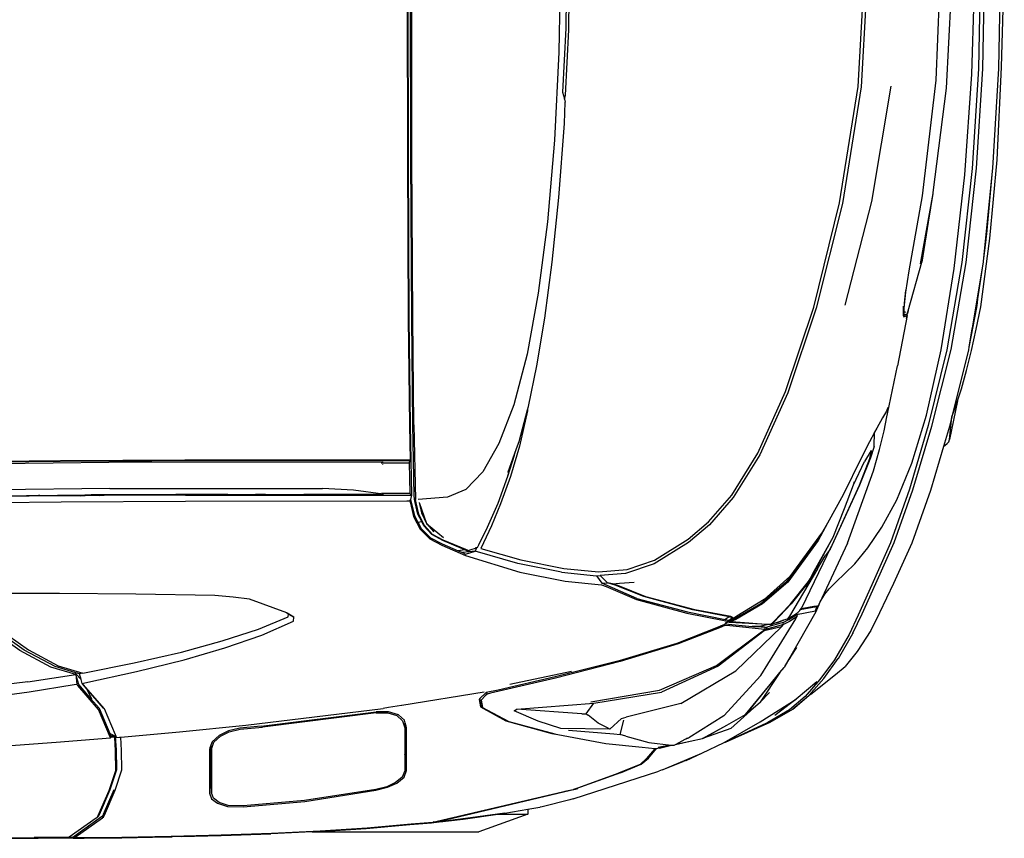
# Model space of a CAD drawing. Units: inches. Extents: x 22042254 to 25404563, y 17568978 to 17626777.
# Tile 7 of 45: x 22042256.1597 to 22042256.7839, y 17568977.6632 to 17568978.1821. Entities that reach past the tile are written whole.
import ezdxf

# ---------------------------------------------------------------- set-up
doc = ezdxf.new("R2010")
doc.units = ezdxf.units.IN
doc.header["$MEASUREMENT"] = 0
doc.layers.add('A-SITE-VEHI', color=8, linetype='Continuous', lineweight=18)
doc.layers.add('Edges', color=250, linetype='Continuous')

# ---------------------------------------------------------------- blocks, each defined once
blk = doc.blocks.new('Nissan Qashqai pl')
at = {"layer": 'Edges'}
for p, q in [((10.6151, 12.8159), (10.6644, 12.8162)), ((10.6176, 12.8164), (10.6651, 12.8167)), ((10.6644, 12.8162), (10.7078, 12.8159)), ((10.6651, 12.8167), (10.666, 12.8167)), ((10.666, 12.8167), (10.677, 12.8167)), ((10.6729, 12.8157), (10.7082, 12.8156)), ((10.6809, 12.8167), (10.677, 12.8167)), ((10.7128, 12.8166), (10.6809, 12.8167)), ((10.7078, 12.8159), (10.7083, 12.8156)), ((10.7082, 12.8156), (10.7078, 12.8159)), ((10.7085, 12.8153), (10.7082, 12.8156)), ((10.7082, 12.8156), (10.7083, 12.8156)), ((10.7083, 12.8156), (10.7087, 12.8153)), ((10.7083, 12.8156), (10.7125, 12.8156)), ((10.7087, 12.8153), (10.7363, 12.7959)), ((10.7139, 12.8164), (10.7125, 12.8156)), ((10.7137, 12.8148), (10.7125, 12.8156)), ((10.7128, 12.8166), (10.7625, 12.8161)), ((10.7128, 12.8166), (10.724, 12.8166)), ((10.7139, 12.8164), (10.7148, 12.8157)), ((10.7628, 12.8158), (10.7139, 12.8164)), ((10.7148, 12.8157), (10.7429, 12.7956)), ((10.7685, 12.8161), (10.724, 12.8166)), ((10.7625, 12.8161), (10.7628, 12.8161)), ((10.7628, 12.8161), (10.8099, 12.8152)), ((10.8131, 12.8149), (10.7628, 12.8158)), ((10.7688, 12.8161), (10.7685, 12.8161)), ((10.8099, 12.8152), (10.7688, 12.8161)), ((10.8099, 12.8152), (10.8131, 12.8152)), ((10.8134, 12.8152), (10.8131, 12.8152)), ((10.8134, 12.8152), (10.8142, 12.8152)), ((10.8142, 12.8152), (10.8142, 12.8152)), ((10.8237, 12.8149), (10.8142, 12.8152)), ((10.7137, 12.8148), (10.7138, 12.8147)), ((10.7418, 12.7947), (10.7138, 12.8147)), ((10.8644, 12.8135), (10.8131, 12.8149)), ((10.8237, 12.8149), (10.864, 12.8138)), ((10.8596, 12.8138), (10.8589, 12.8138)), ((10.8642, 12.8136), (10.8596, 12.8138)), ((10.864, 12.8138), (10.8642, 12.8138)), ((10.8642, 12.8138), (10.9152, 12.812)), ((10.9158, 12.8118), (10.8644, 12.8135)), ((10.9577, 12.8101), (10.9152, 12.812)), ((10.9657, 12.8095), (10.9158, 12.8118)), ((10.9577, 12.8101), (10.9649, 12.8097)), ((10.9577, 12.8101), (11.1283, 12.8101)), ((10.9649, 12.8097), (11.0127, 12.8067)), ((11.0138, 12.8064), (10.9657, 12.8095)), ((11.0127, 12.8067), (11.0576, 12.8026)), ((11.059, 12.8023), (11.0138, 12.8064)), ((11.1783, 12.7921), (11.1283, 12.8101)), ((10.7363, 12.7959), (10.7376, 12.795)), ((10.7387, 12.794), (10.7376, 12.795)), ((10.7376, 12.795), (10.7378, 12.7946)), ((10.7432, 12.7954), (10.7426, 12.7954)), ((10.7429, 12.7956), (10.7432, 12.7954)), ((10.7441, 12.7954), (10.7432, 12.7954)), ((10.7432, 12.7954), (10.744, 12.7948)), ((11.0576, 12.8026), (11.0798, 12.8008)), ((11.0768, 12.8008), (11.059, 12.8023)), ((11.0811, 12.8004), (11.0768, 12.8008)), ((11.0798, 12.8008), (11.0872, 12.7999)), ((11.0827, 12.8001), (11.0811, 12.8004)), ((11.0827, 12.8001), (11.0813, 12.7998)), ((11.0836, 12.8002), (11.0827, 12.8001)), ((11.0856, 12.7994), (11.0827, 12.8001)), ((11.0872, 12.7999), (11.0836, 12.8002)), ((11.0836, 12.8002), (11.0882, 12.7992)), ((11.2196, 12.7681), (11.0856, 12.7994)), ((11.0883, 12.7998), (11.0872, 12.7999)), ((11.0882, 12.7992), (11.2222, 12.7676)), ((11.0883, 12.7998), (11.1123, 12.797)), ((11.1147, 12.7965), (11.0883, 12.7998)), ((11.1123, 12.797), (11.1475, 12.7921)), ((11.1547, 12.791), (11.1147, 12.7965)), ((10.7378, 12.7946), (10.7379, 12.7945)), ((10.7378, 12.7946), (10.7385, 12.7932)), ((10.7385, 12.7932), (10.7497, 12.7679)), ((10.7387, 12.794), (10.7396, 12.7922)), ((10.7396, 12.7922), (10.7507, 12.7669)), ((10.743, 12.7939), (10.7418, 12.7947)), ((10.7434, 12.793), (10.743, 12.7939)), ((10.7437, 12.7921), (10.7434, 12.793)), ((10.7438, 12.7921), (10.7437, 12.7921)), ((10.7438, 12.7921), (10.7549, 12.7666)), ((10.744, 12.7948), (10.7448, 12.793)), ((10.7448, 12.793), (10.7559, 12.7674)), ((11.1475, 12.7921), (11.1525, 12.7914)), ((11.1475, 12.7921), (11.1783, 12.7921)), ((11.1525, 12.7914), (11.1547, 12.791)), ((11.1547, 12.791), (11.1783, 12.787)), ((11.1783, 12.787), (11.1783, 12.7921)), ((11.1783, 12.787), (11.1906, 12.7849)), ((11.1906, 12.7849), (11.1909, 12.7849)), ((11.193, 12.7845), (11.1909, 12.7849)), ((10.8523, 12.7704), (10.8546, 12.7762)), ((10.8565, 12.7757), (10.8543, 12.7702)), ((10.8546, 12.7762), (10.8607, 12.7808)), ((10.8622, 12.7801), (10.8565, 12.7757)), ((10.8607, 12.7808), (10.8708, 12.7841)), ((10.8716, 12.7832), (10.8622, 12.7801)), ((10.8708, 12.7841), (10.8869, 12.7844)), ((10.887, 12.7835), (10.8716, 12.7832)), ((10.8869, 12.7844), (10.9499, 12.7789)), ((10.9498, 12.7781), (10.887, 12.7835)), ((11.0226, 12.7668), (10.9498, 12.7781)), ((10.9499, 12.7789), (11.0229, 12.7676)), ((11.2215, 12.7775), (11.193, 12.7845)), ((11.2247, 12.7764), (11.2215, 12.7775)), ((11.2247, 12.7764), (11.3124, 12.7479)), ((10.7497, 12.7679), (10.7565, 12.7473)), ((10.7507, 12.7669), (10.7575, 12.7462)), ((10.7559, 12.7674), (10.7626, 12.7467)), ((10.8523, 12.7255), (10.8523, 12.7704)), ((10.8543, 12.7702), (10.8538, 12.753)), ((10.8543, 12.7255), (10.8543, 12.7702)), ((11.0339, 12.7639), (11.0226, 12.7668)), ((11.0229, 12.7676), (11.0348, 12.7645)), ((11.2247, 12.767), (11.2163, 12.7689)), ((11.22, 12.768), (11.2196, 12.7681)), ((11.2247, 12.767), (11.22, 12.768)), ((11.2222, 12.7676), (11.2271, 12.7664)), ((11.2253, 12.7668), (11.2247, 12.767)), ((11.2304, 12.7649), (11.2253, 12.7668)), ((11.2253, 12.7668), (11.2271, 12.7664)), ((11.2271, 12.7664), (11.2296, 12.7658)), ((11.2271, 12.7664), (11.2277, 12.7662)), ((11.2277, 12.7662), (11.2296, 12.7658)), ((11.2732, 12.7496), (11.2277, 12.7662)), ((11.2704, 12.7504), (11.2304, 12.7649)), ((11.0429, 12.7597), (11.0339, 12.7639)), ((11.0348, 12.7645), (11.0444, 12.7601)), ((11.0497, 12.7542), (11.0429, 12.7597)), ((11.0444, 12.7601), (11.0516, 12.7542)), ((10.7565, 12.7473), (10.7563, 12.7273)), ((10.7575, 12.7462), (10.7572, 12.7263)), ((10.7626, 12.7467), (10.7623, 12.7269)), ((10.8528, 12.7503), (10.8535, 12.7521)), ((10.8528, 12.742), (10.8528, 12.7503)), ((10.8535, 12.7521), (10.8538, 12.753)), ((10.8538, 12.7521), (10.8535, 12.7521)), ((10.8538, 12.753), (10.8538, 12.7521)), ((10.8538, 12.7521), (10.8538, 12.7502)), ((10.8538, 12.7502), (10.8538, 12.742)), ((11.0523, 12.7475), (11.0497, 12.7542)), ((11.0516, 12.7542), (11.0543, 12.7473)), ((11.0528, 12.73), (11.0523, 12.7475)), ((11.0523, 12.7312), (11.0523, 12.7475)), ((11.0543, 12.7473), (11.0543, 12.7035)), ((11.2702, 12.7507), (11.2704, 12.7504)), ((11.2704, 12.7506), (11.2707, 12.7503)), ((11.2707, 12.7503), (11.2704, 12.7504)), ((11.2719, 12.7498), (11.2707, 12.7503)), ((11.2934, 12.741), (11.2719, 12.7498)), ((11.2732, 12.7496), (11.2946, 12.7409)), ((11.3161, 12.7467), (11.3124, 12.7479)), ((11.3161, 12.7467), (11.3376, 12.7381)), ((11.3192, 12.7454), (11.3566, 12.7294)), ((10.8528, 12.742), (10.8538, 12.742)), ((10.8528, 12.7419), (10.8528, 12.742)), ((10.8538, 12.7419), (10.8528, 12.7419)), ((10.8528, 12.7242), (10.8528, 12.7419)), ((10.8538, 12.742), (10.8538, 12.7419)), ((10.8538, 12.7214), (10.8538, 12.7419)), ((11.3, 12.735), (11.2934, 12.741)), ((11.2946, 12.7409), (11.3018, 12.7346)), ((11.3081, 12.7253), (11.3, 12.735)), ((11.3018, 12.7346), (11.3103, 12.7249)), ((11.3405, 12.7369), (11.3376, 12.7381)), ((11.3405, 12.7369), (11.3566, 12.7294)), ((10.7563, 12.7273), (10.7553, 12.7134)), ((10.7572, 12.7263), (10.7563, 12.7126)), ((10.7623, 12.7269), (10.7615, 12.7131)), ((10.8528, 12.7242), (10.8523, 12.7255)), ((10.8543, 12.7255), (10.8569, 12.7184)), ((11.0523, 12.7312), (11.0528, 12.73)), ((11.0523, 12.7287), (11.0523, 12.7312)), ((11.0528, 12.7274), (11.0523, 12.7287)), ((11.0523, 12.7037), (11.0523, 12.7287)), ((11.0528, 12.7274), (11.0528, 12.73)), ((11.0528, 12.73), (11.0538, 12.7273)), ((11.0528, 12.7274), (11.0528, 12.6985)), ((11.0538, 12.7273), (11.0538, 12.7018)), ((11.2956, 12.7234), (11.3085, 12.7247)), ((11.3086, 12.7247), (11.3081, 12.7253)), ((11.3081, 12.7253), (11.3087, 12.7247)), ((11.3085, 12.7247), (11.3086, 12.7247)), ((11.3086, 12.7247), (11.3087, 12.7247)), ((11.3087, 12.7247), (11.3103, 12.7249)), ((11.3103, 12.7249), (11.3103, 12.7249)), ((11.3103, 12.7249), (11.3106, 12.7249)), ((11.3106, 12.7249), (11.314, 12.7238)), ((11.3566, 12.7294), (11.3796, 12.7187)), ((10.6318, 12.7228), (10.6955, 12.7184)), ((10.6955, 12.7184), (10.7509, 12.714)), ((10.8538, 12.7214), (10.8528, 12.7242)), ((10.855, 12.7181), (10.8538, 12.7214)), ((10.8622, 12.7114), (10.855, 12.7181)), ((10.8569, 12.7184), (10.8637, 12.712)), ((11.2091, 12.7103), (11.2583, 12.7196)), ((11.2583, 12.7196), (11.2956, 12.7234)), ((11.2787, 12.7123), (11.3022, 12.7186)), ((11.3022, 12.7186), (11.3252, 12.7213)), ((11.317, 12.7227), (11.3119, 12.7236)), ((11.3132, 12.7243), (11.3256, 12.7215)), ((11.314, 12.7238), (11.317, 12.7227)), ((11.314, 12.7238), (11.3242, 12.7216)), ((11.3242, 12.7216), (11.317, 12.7227)), ((11.3198, 12.7211), (11.3252, 12.7213)), ((11.3242, 12.7216), (11.3256, 12.7215)), ((11.3252, 12.7213), (11.3283, 12.7214)), ((11.3256, 12.7215), (11.3283, 12.7214)), ((11.3283, 12.7214), (11.3297, 12.7206)), ((11.3297, 12.7206), (11.3446, 12.7173)), ((11.3297, 12.7206), (11.3302, 12.7203)), ((11.3302, 12.7203), (11.3446, 12.7173)), ((11.3302, 12.7203), (11.3394, 12.7152)), ((11.3394, 12.7152), (11.3434, 12.7138)), ((11.3394, 12.7152), (11.342, 12.7137)), ((11.3446, 12.7173), (11.3571, 12.7146)), ((11.3583, 12.7142), (11.3571, 12.7146)), ((11.3571, 12.7146), (11.3821, 12.7008)), ((11.3796, 12.7187), (11.4164, 12.6974)), ((11.3796, 12.7187), (11.3807, 12.7182)), ((11.3807, 12.7182), (11.4267, 12.6979)), ((11.4228, 12.6989), (11.3807, 12.7182)), ((10.7501, 12.7114), (10.7387, 12.6849)), ((10.7507, 12.7098), (10.7397, 12.684)), ((10.7563, 12.7109), (10.7449, 12.6843)), ((10.7507, 12.7132), (10.7501, 12.7114)), ((10.7506, 12.7111), (10.7507, 12.7132)), ((10.7507, 12.7132), (10.7509, 12.714)), ((10.751, 12.7132), (10.7507, 12.7132)), ((10.7511, 12.7107), (10.7507, 12.7098)), ((10.7524, 12.7106), (10.7507, 12.7098)), ((10.7522, 12.7131), (10.7509, 12.714)), ((10.7516, 12.7131), (10.7509, 12.714)), ((10.7519, 12.7128), (10.7511, 12.7107)), ((10.7522, 12.7131), (10.7516, 12.7131)), ((10.7519, 12.7128), (10.7516, 12.7131)), ((10.7526, 12.7124), (10.7519, 12.7128)), ((10.7553, 12.7134), (10.7522, 12.7131)), ((10.7524, 12.7106), (10.7526, 12.7124)), ((10.7556, 12.7122), (10.7524, 12.7106)), ((10.7526, 12.7124), (10.7526, 12.7127)), ((10.7532, 12.712), (10.7526, 12.7124)), ((10.7556, 12.7122), (10.7532, 12.712)), ((10.7561, 12.7125), (10.7556, 12.7122)), ((10.7561, 12.7125), (10.7563, 12.7126)), ((10.7563, 12.7125), (10.7561, 12.7125)), ((10.7563, 12.7123), (10.7561, 12.7123)), ((10.7563, 12.7126), (10.7573, 12.7135)), ((10.7563, 12.7126), (10.7563, 12.7125)), ((10.7569, 12.7125), (10.7563, 12.7109)), ((10.7569, 12.7125), (10.7563, 12.7125)), ((10.7563, 12.7125), (10.7563, 12.7123)), ((10.7573, 12.7135), (10.7569, 12.7125)), ((10.7573, 12.7135), (10.7604, 12.7132)), ((10.7604, 12.7132), (10.7615, 12.7131)), ((10.7615, 12.7131), (10.8218, 12.7077)), ((10.8218, 12.7077), (10.8896, 12.7008)), ((10.8718, 12.7068), (10.8622, 12.7114)), ((10.8637, 12.712), (10.8727, 12.7077)), ((10.8836, 12.7041), (10.8718, 12.7068)), ((10.8727, 12.7077), (10.8839, 12.7051)), ((10.8839, 12.7051), (10.9067, 12.7029)), ((11.156, 12.6966), (11.203, 12.7093)), ((11.1589, 12.6971), (11.2062, 12.7098)), ((11.2121, 12.7043), (11.189, 12.6968)), ((11.203, 12.7093), (11.2091, 12.7103)), ((11.2062, 12.7098), (11.2091, 12.7103)), ((11.2622, 12.7051), (11.2121, 12.7043)), ((11.2199, 12.706), (11.2666, 12.7097)), ((11.2622, 12.7051), (11.2601, 12.7037)), ((11.2743, 12.6942), (11.2622, 12.7051)), ((11.2666, 12.7097), (11.2729, 12.7104)), ((11.2787, 12.7123), (11.2729, 12.7104)), ((11.2729, 12.7104), (11.2766, 12.6957)), ((11.379, 12.6915), (11.3434, 12.7138)), ((11.3583, 12.7142), (11.3821, 12.7008)), ((11.3864, 12.7044), (11.3583, 12.7142)), ((11.4163, 12.6775), (11.3864, 12.7044)), ((10.9054, 12.702), (10.8836, 12.7041)), ((10.8896, 12.7008), (11.0304, 12.6838)), ((10.9054, 12.702), (11.0232, 12.6871)), ((11.0231, 12.6882), (10.9067, 12.7029)), ((11.0443, 12.6911), (11.0501, 12.6964)), ((11.052, 12.6958), (11.0458, 12.6903)), ((11.0501, 12.6964), (11.0523, 12.7037)), ((11.0528, 12.6985), (11.052, 12.6958)), ((11.0538, 12.7018), (11.0528, 12.6985)), ((11.0543, 12.7035), (11.0538, 12.7018)), ((11.1298, 12.6823), (11.156, 12.6966)), ((11.1365, 12.6851), (11.1589, 12.6971)), ((11.189, 12.6968), (11.1644, 12.6862)), ((11.2505, 12.6987), (11.2401, 12.6908)), ((11.2601, 12.7037), (11.2505, 12.6987)), ((11.2743, 12.6942), (11.2791, 12.6927)), ((11.3821, 12.7008), (11.4014, 12.69)), ((11.4164, 12.6974), (11.4531, 12.6744)), ((11.4243, 12.6982), (11.4228, 12.6989)), ((11.4464, 12.6853), (11.4243, 12.6982)), ((11.4267, 12.6979), (11.4498, 12.6844)), ((10.7387, 12.6849), (10.7177, 12.6604)), ((10.7449, 12.6843), (10.7232, 12.6594)), ((11.0231, 12.6882), (11.035, 12.6883)), ((11.0358, 12.6872), (11.0232, 12.6871)), ((11.035, 12.6883), (11.0443, 12.6911)), ((11.0458, 12.6903), (11.0358, 12.6872)), ((11.1319, 12.6827), (11.1365, 12.6851)), ((11.1644, 12.6862), (11.1672, 12.6844)), ((11.2337, 12.6892), (11.1672, 12.6844)), ((11.1672, 12.6844), (11.2459, 12.6785)), ((11.2337, 12.6892), (11.2382, 12.6892)), ((11.2382, 12.6892), (11.2401, 12.6908)), ((11.2382, 12.6892), (11.2459, 12.6785)), ((11.335, 12.6786), (11.2791, 12.6927)), ((11.379, 12.6915), (11.417, 12.6499)), ((11.4014, 12.69), (11.4022, 12.6894)), ((11.4014, 12.69), (11.4265, 12.6594)), ((11.4022, 12.6894), (11.4163, 12.6775)), ((11.4022, 12.6894), (11.4265, 12.6594)), ((11.4531, 12.6744), (11.4314, 12.6911)), ((11.4624, 12.6717), (11.4464, 12.6853)), ((11.4498, 12.6844), (11.4662, 12.6706)), ((11.4681, 12.6691), (11.4498, 12.6844)), ((10.6678, 12.6672), (10.6152, 12.674)), ((10.7334, 12.6766), (10.7186, 12.6593)), ((10.7438, 12.6836), (10.7265, 12.6635)), ((10.7265, 12.6635), (10.7316, 12.6741)), ((10.7397, 12.684), (10.7334, 12.6766)), ((11.0357, 12.6829), (11.0304, 12.6838)), ((11.0491, 12.6807), (11.0357, 12.6829)), ((11.0449, 12.6812), (11.0448, 12.6812)), ((11.0492, 12.6807), (11.0491, 12.6807)), ((11.1336, 12.667), (11.0492, 12.6807)), ((11.1285, 12.6745), (11.1298, 12.6823)), ((11.1293, 12.6736), (11.1285, 12.6745)), ((11.1306, 12.6812), (11.1293, 12.6736)), ((11.1306, 12.6752), (11.1319, 12.6827)), ((11.1319, 12.6827), (11.1306, 12.6812)), ((11.1347, 12.671), (11.1306, 12.6752)), ((11.2428, 12.6769), (11.3132, 12.6652)), ((11.2459, 12.6785), (11.3153, 12.6672)), ((11.335, 12.6786), (11.3915, 12.6453)), ((11.4366, 12.6471), (11.4163, 12.6775)), ((11.4163, 12.6775), (11.4259, 12.6674)), ((11.4742, 12.6567), (11.4531, 12.6744)), ((10.7137, 12.6595), (10.6678, 12.6672)), ((11.1353, 12.6677), (11.1293, 12.6736)), ((11.1366, 12.6691), (11.1347, 12.671)), ((11.1358, 12.6676), (11.1353, 12.6677)), ((11.1358, 12.6676), (11.1366, 12.6691)), ((11.148, 12.665), (11.1358, 12.6676)), ((11.1401, 12.6682), (11.1366, 12.6691)), ((11.2066, 12.6527), (11.1401, 12.6682)), ((11.2063, 12.6515), (11.148, 12.665)), ((11.3132, 12.6652), (11.3715, 12.6398)), ((11.3733, 12.6404), (11.3153, 12.6672)), ((11.4774, 12.6543), (11.4624, 12.6717)), ((11.4662, 12.6706), (11.4815, 12.6531)), ((11.4681, 12.6691), (11.4936, 12.6491)), ((10.6664, 12.6566), (10.6144, 12.6629)), ((10.6664, 12.6566), (10.7155, 12.649)), ((10.7165, 12.6591), (10.7137, 12.6595)), ((10.7186, 12.6593), (10.7155, 12.649)), ((10.7155, 12.649), (10.7165, 12.6591)), ((10.7209, 12.654), (10.7155, 12.6485)), ((10.7177, 12.6604), (10.7165, 12.6591)), ((10.7209, 12.654), (10.7192, 12.6484)), ((10.7221, 12.6581), (10.7209, 12.654)), ((10.7232, 12.6594), (10.7221, 12.6581)), ((10.7221, 12.6581), (10.7224, 12.6587)), ((10.7221, 12.6581), (10.7247, 12.6575)), ((10.7265, 12.6635), (10.7224, 12.6587)), ((10.7247, 12.6575), (10.7776, 12.646)), ((11.2232, 12.6458), (11.1598, 12.6594)), ((11.4265, 12.6594), (11.4366, 12.6471)), ((11.4924, 12.6339), (11.4774, 12.6543)), ((10.7155, 12.649), (10.69, 12.6414)), ((10.7155, 12.6473), (10.6943, 12.641)), ((10.6976, 12.6401), (10.7228, 12.6477)), ((10.7155, 12.649), (10.7155, 12.6485)), ((10.7155, 12.6485), (10.7155, 12.6473)), ((10.7192, 12.6484), (10.7155, 12.6473)), ((10.7228, 12.6477), (10.7192, 12.6484)), ((10.7228, 12.6477), (10.7754, 12.637)), ((10.7776, 12.646), (10.8264, 12.6341)), ((11.272, 12.6349), (11.2063, 12.6515)), ((11.2728, 12.6357), (11.2066, 12.6527)), ((11.3915, 12.6453), (11.4381, 12.6002)), ((11.417, 12.6499), (11.4529, 12.5922)), ((11.4366, 12.6471), (11.4408, 12.6419)), ((11.4815, 12.6531), (11.4963, 12.6328)), ((11.4936, 12.6491), (11.5033, 12.6408)), ((10.69, 12.6414), (10.6583, 12.6245)), ((10.6943, 12.641), (10.6627, 12.6241)), ((10.6671, 12.6238), (10.6976, 12.6401)), ((10.7754, 12.637), (10.8239, 12.6261)), ((10.8264, 12.6341), (10.8682, 12.6216)), ((11.3311, 12.6172), (11.272, 12.6349)), ((11.3323, 12.6178), (11.2728, 12.6357)), ((11.3715, 12.6398), (11.4177, 12.6052)), ((11.4203, 12.6044), (11.3733, 12.6404)), ((11.4408, 12.6419), (11.4411, 12.6414)), ((11.4411, 12.6414), (11.4411, 12.6414)), ((11.4414, 12.6409), (11.4411, 12.6414)), ((11.4414, 12.6409), (11.447, 12.6315)), ((11.4455, 12.6336), (11.4414, 12.6409)), ((11.5074, 12.608), (11.4924, 12.6339)), ((11.5158, 12.6256), (11.5033, 12.6408)), ((10.6583, 12.6245), (10.6215, 12.5986)), ((10.6627, 12.6241), (10.6261, 12.5984)), ((10.6306, 12.5982), (10.6671, 12.6238)), ((10.8239, 12.6261), (10.8653, 12.6144)), ((11.447, 12.6315), (11.4455, 12.6336)), ((11.4455, 12.6336), (11.4462, 12.6324)), ((11.447, 12.6315), (11.4462, 12.6324)), ((11.4732, 12.585), (11.4462, 12.6324)), ((11.447, 12.6315), (11.447, 12.6314)), ((11.4536, 12.6215), (11.447, 12.6314)), ((11.4964, 12.6326), (11.4963, 12.6328)), ((11.4964, 12.6326), (11.5113, 12.6069)), ((11.5295, 12.6041), (11.5158, 12.6256)), ((10.8653, 12.6144), (10.9026, 12.6025)), ((10.8682, 12.6216), (10.9059, 12.6087)), ((11.3751, 12.5999), (11.3311, 12.6172)), ((11.3747, 12.6011), (11.3323, 12.6178)), ((10.9059, 12.6087), (10.9384, 12.5945)), ((11.4177, 12.6052), (11.4193, 12.6042)), ((11.4192, 12.6045), (11.4194, 12.6042)), ((11.4194, 12.6042), (11.4193, 12.6042)), ((11.4193, 12.6042), (11.4196, 12.604)), ((11.4194, 12.6042), (11.4196, 12.604)), ((11.4196, 12.6042), (11.4194, 12.6042)), ((11.4196, 12.604), (11.4201, 12.6036)), ((11.4198, 12.6041), (11.4201, 12.6036)), ((11.4201, 12.6036), (11.4212, 12.603)), ((11.4292, 12.6024), (11.4203, 12.6044)), ((11.4229, 12.6025), (11.4203, 12.6044)), ((11.5165, 12.5882), (11.5074, 12.608)), ((11.5113, 12.6068), (11.5113, 12.6069)), ((11.5113, 12.6068), (11.5206, 12.5869)), ((11.5384, 12.5859), (11.5295, 12.6041)), ((10.9026, 12.6025), (10.933, 12.5901)), ((10.9384, 12.5945), (10.9386, 12.5905)), ((11.3411, 12.5863), (11.3795, 12.5939)), ((11.38, 12.5988), (11.3747, 12.6011)), ((11.3751, 12.5999), (11.3762, 12.5999)), ((11.3752, 12.5998), (11.3751, 12.5999)), ((11.3763, 12.5998), (11.3752, 12.5998)), ((11.3764, 12.5993), (11.3752, 12.5998)), ((11.3792, 12.5982), (11.3764, 12.5993)), ((11.3792, 12.5982), (11.3793, 12.5979)), ((11.3792, 12.5982), (11.3804, 12.5972)), ((11.3795, 12.5939), (11.3834, 12.5947)), ((11.3853, 12.5993), (11.38, 12.5988)), ((11.3804, 12.5972), (11.4082, 12.5998)), ((11.3827, 12.5953), (11.3804, 12.5972)), ((11.3804, 12.5926), (11.3841, 12.5933)), ((11.3811, 12.5958), (11.3808, 12.5961)), ((11.3834, 12.5947), (11.3827, 12.5953)), ((11.3846, 12.5953), (11.3829, 12.5952)), ((11.3829, 12.5952), (11.3849, 12.5951)), ((11.388, 12.591), (11.3829, 12.5952)), ((11.3834, 12.5947), (11.3841, 12.5933)), ((11.3846, 12.5953), (11.4248, 12.5976)), ((11.3846, 12.5953), (11.3846, 12.5953)), ((11.3851, 12.5951), (11.3846, 12.5953)), ((11.3846, 12.5953), (11.3849, 12.5951)), ((11.3849, 12.5951), (11.3851, 12.5951)), ((11.3882, 12.5923), (11.3849, 12.5951)), ((11.3851, 12.5951), (11.3867, 12.5949)), ((11.4171, 12.5766), (11.3851, 12.5951)), ((11.4212, 12.603), (11.3853, 12.5993)), ((11.3867, 12.5949), (11.3915, 12.5951)), ((11.3914, 12.5926), (11.3867, 12.5949)), ((11.3915, 12.5951), (11.4266, 12.5977)), ((11.409, 12.5999), (11.4082, 12.5998)), ((11.4164, 12.5998), (11.4082, 12.5998)), ((11.4152, 12.6004), (11.409, 12.5999)), ((11.409, 12.5999), (11.4163, 12.5999)), ((11.4173, 12.6006), (11.4152, 12.6004)), ((11.4163, 12.5999), (11.4152, 12.6004)), ((11.4163, 12.5999), (11.4186, 12.5999)), ((11.4164, 12.5998), (11.4163, 12.5999)), ((11.4181, 12.5998), (11.4164, 12.5998)), ((11.4169, 12.5996), (11.4164, 12.5998)), ((11.4252, 12.598), (11.4169, 12.5996)), ((11.4176, 12.6007), (11.4173, 12.6006)), ((11.418, 12.6006), (11.4173, 12.6006)), ((11.4215, 12.601), (11.4176, 12.6007)), ((11.418, 12.6006), (11.4176, 12.6007)), ((11.4204, 12.6002), (11.418, 12.6006)), ((11.4194, 12.6), (11.418, 12.6006)), ((11.4212, 12.603), (11.4215, 12.601)), ((11.4218, 12.6028), (11.4212, 12.603)), ((11.4215, 12.601), (11.4219, 12.6009)), ((11.4222, 12.6029), (11.4218, 12.6028)), ((11.4229, 12.6025), (11.4218, 12.6028)), ((11.4219, 12.6009), (11.4222, 12.6005)), ((11.4219, 12.6009), (11.4224, 12.6008)), ((11.4224, 12.6008), (11.4226, 12.6006)), ((11.4224, 12.6008), (11.423, 12.6006)), ((11.4315, 12.6002), (11.4229, 12.6025)), ((11.423, 12.6006), (11.4229, 12.6025)), ((11.44, 12.5959), (11.423, 12.6006)), ((11.4248, 12.5976), (11.4266, 12.5977)), ((11.4266, 12.5977), (11.4252, 12.598)), ((11.4266, 12.5977), (11.4268, 12.5977)), ((11.4268, 12.5977), (11.4296, 12.5954)), ((11.4268, 12.5977), (11.4278, 12.5977)), ((11.4303, 12.5956), (11.4278, 12.5977)), ((11.4278, 12.5977), (11.43, 12.5969)), ((11.4381, 12.6002), (11.4292, 12.6024)), ((11.4296, 12.5954), (11.4469, 12.5773)), ((11.4337, 12.5962), (11.43, 12.5969)), ((11.43, 12.5969), (11.4361, 12.5948)), ((11.4479, 12.5766), (11.4303, 12.5956)), ((11.4403, 12.5978), (11.4315, 12.6002)), ((11.4397, 12.5937), (11.4337, 12.5962)), ((11.4361, 12.5948), (11.4406, 12.5932)), ((11.4381, 12.6002), (11.4403, 12.5978)), ((11.4406, 12.5932), (11.4397, 12.5937)), ((11.4403, 12.5978), (11.44, 12.5959)), ((11.44, 12.5959), (11.4457, 12.5928)), ((11.4462, 12.5947), (11.4403, 12.5978)), ((11.452, 12.591), (11.4462, 12.5947)), ((10.9316, 12.586), (10.8932, 12.572)), ((10.9316, 12.586), (10.9334, 12.5872)), ((10.932, 12.5862), (10.9316, 12.586)), ((10.9335, 12.5871), (10.932, 12.5862)), ((10.933, 12.5901), (10.9334, 12.5872)), ((10.9334, 12.5872), (10.9386, 12.5905)), ((10.9334, 12.5872), (10.9335, 12.5871)), ((10.9386, 12.5905), (10.9335, 12.5871)), ((11.2895, 12.5724), (11.3411, 12.5863)), ((11.29, 12.5711), (11.3419, 12.585)), ((11.3419, 12.585), (11.3804, 12.5926)), ((11.3847, 12.5899), (11.3474, 12.5827)), ((11.3863, 12.5898), (11.3493, 12.5828)), ((11.3847, 12.5899), (11.3804, 12.5926)), ((11.3847, 12.5899), (11.3848, 12.5899)), ((11.388, 12.591), (11.3848, 12.5899)), ((11.3895, 12.5912), (11.3863, 12.5898)), ((11.3886, 12.5919), (11.3872, 12.5927)), ((11.3882, 12.5923), (11.3886, 12.5919)), ((11.3886, 12.5919), (11.3895, 12.5912)), ((11.3892, 12.5916), (11.3886, 12.5919)), ((11.3923, 12.5894), (11.3895, 12.5912)), ((11.4187, 12.5768), (11.3914, 12.5926)), ((11.4203, 12.5724), (11.3923, 12.5894)), ((11.4406, 12.5932), (11.4442, 12.592)), ((11.4442, 12.592), (11.4497, 12.589)), ((11.4462, 12.5893), (11.4442, 12.592)), ((11.4457, 12.5928), (11.4512, 12.5893)), ((11.475, 12.5409), (11.4462, 12.5893)), ((11.4497, 12.589), (11.4498, 12.5889)), ((11.4535, 12.5876), (11.4498, 12.5889)), ((11.4498, 12.5889), (11.4549, 12.5855)), ((11.4512, 12.5893), (11.4535, 12.5876)), ((11.4539, 12.5897), (11.452, 12.591)), ((11.4529, 12.5922), (11.4542, 12.5894)), ((11.4535, 12.5876), (11.4532, 12.5882)), ((11.4535, 12.5876), (11.4542, 12.5894)), ((11.4535, 12.5876), (11.4728, 12.5838)), ((11.4542, 12.5894), (11.4539, 12.5897)), ((11.4549, 12.5855), (11.4568, 12.5836)), ((11.4564, 12.5833), (11.4567, 12.5833)), ((11.4568, 12.5836), (11.4571, 12.5833)), ((11.4571, 12.5833), (11.4573, 12.583)), ((11.4732, 12.585), (11.4728, 12.5838)), ((11.4728, 12.5838), (11.4742, 12.5797)), ((11.4728, 12.5838), (11.4746, 12.5796)), ((11.4758, 12.5791), (11.4732, 12.585)), ((11.5306, 12.5573), (11.5165, 12.5882)), ((11.5206, 12.5869), (11.5349, 12.5559)), ((11.5527, 12.5559), (11.5384, 12.5859)), ((11.3474, 12.5827), (11.2972, 12.5692)), ((11.3493, 12.5828), (11.2993, 12.5695)), ((11.3474, 12.5827), (11.3474, 12.5827)), ((11.4433, 12.5543), (11.4171, 12.5766)), ((11.4447, 12.5545), (11.4187, 12.5768)), ((11.4469, 12.5773), (11.4659, 12.5539)), ((11.4654, 12.5548), (11.4479, 12.5766)), ((11.4569, 12.583), (11.4565, 12.5831)), ((11.4573, 12.583), (11.4578, 12.5822)), ((11.4704, 12.5803), (11.4573, 12.583)), ((11.4573, 12.5823), (11.4574, 12.5822)), ((11.4573, 12.5823), (11.4573, 12.5823)), ((11.4576, 12.5822), (11.4574, 12.5822)), ((11.4578, 12.5822), (11.4588, 12.5807)), ((11.4605, 12.5816), (11.4578, 12.5822)), ((11.4588, 12.5807), (11.4895, 12.5178)), ((11.4713, 12.5794), (11.4605, 12.5816)), ((11.4742, 12.5797), (11.4704, 12.5803)), ((11.4744, 12.5792), (11.4713, 12.5794)), ((11.4742, 12.5797), (11.4744, 12.5792)), ((11.4745, 12.5797), (11.4742, 12.5797)), ((11.4745, 12.5792), (11.4744, 12.5792)), ((11.4745, 12.5792), (11.4745, 12.5797)), ((11.4745, 12.5797), (11.4746, 12.5796)), ((11.4748, 12.5792), (11.4745, 12.5792)), ((11.4746, 12.5796), (11.4748, 12.5792)), ((11.4746, 12.5796), (11.4758, 12.5791)), ((11.4758, 12.5791), (11.4748, 12.5792)), ((11.4758, 12.5791), (11.4759, 12.579)), ((11.4759, 12.579), (11.4778, 12.5746)), ((11.4759, 12.579), (11.4771, 12.576)), ((11.5057, 12.5145), (11.4771, 12.576)), ((11.4778, 12.5746), (11.4826, 12.5669)), ((10.6988, 12.5662), (10.5892, 12.5659)), ((10.7769, 12.5667), (10.6988, 12.5662)), ((10.858, 12.5683), (10.7769, 12.5667)), ((10.8766, 12.5697), (10.858, 12.5683)), ((10.8932, 12.572), (10.8766, 12.5697)), ((11.29, 12.5711), (11.2541, 12.5557)), ((11.2586, 12.5591), (11.2895, 12.5724)), ((11.2972, 12.5692), (11.2677, 12.5575)), ((11.2993, 12.5695), (11.2705, 12.5579)), ((11.4467, 12.5488), (11.4203, 12.5724)), ((11.4826, 12.5669), (11.4869, 12.5615)), ((11.1702, 12.5444), (11.2166, 12.5534)), ((11.2166, 12.5534), (11.2538, 12.5571)), ((11.2488, 12.548), (11.2541, 12.5557)), ((11.2599, 12.5552), (11.2524, 12.5477)), ((11.2538, 12.5571), (11.2586, 12.5591)), ((11.2541, 12.5557), (11.2599, 12.5552)), ((11.2677, 12.5575), (11.2599, 12.5552)), ((11.265, 12.5563), (11.2599, 12.5552)), ((11.2705, 12.5579), (11.265, 12.5563)), ((11.265, 12.5563), (11.2724, 12.5557)), ((11.2724, 12.5557), (11.2874, 12.5544)), ((11.4745, 12.5116), (11.4433, 12.5543)), ((11.4758, 12.5118), (11.4447, 12.5545)), ((11.4633, 12.5594), (11.4897, 12.5108)), ((11.4654, 12.5548), (11.4659, 12.5539)), ((11.4659, 12.5539), (11.4674, 12.5512)), ((11.4869, 12.5615), (11.4933, 12.555)), ((11.5131, 12.5356), (11.4933, 12.555)), ((11.5496, 12.5141), (11.5306, 12.5573)), ((11.5349, 12.5559), (11.5535, 12.5139)), ((11.5716, 12.5145), (11.5527, 12.5559)), ((11.1144, 12.5271), (11.1702, 12.5444)), ((11.2127, 12.5443), (11.1683, 12.5354)), ((11.2127, 12.5443), (11.2488, 12.548)), ((11.2152, 12.5404), (11.2509, 12.5439)), ((11.2488, 12.548), (11.2524, 12.5477)), ((11.2509, 12.5439), (11.28, 12.5414)), ((11.2785, 12.5455), (11.2524, 12.5477)), ((11.3076, 12.5358), (11.2785, 12.5455)), ((11.4801, 12.503), (11.4467, 12.5488)), ((11.4675, 12.551), (11.4674, 12.5512)), ((11.4675, 12.551), (11.4703, 12.546)), ((11.4703, 12.546), (11.4704, 12.5458)), ((11.4704, 12.5458), (11.4909, 12.5085)), ((11.4704, 12.5458), (11.4897, 12.5108)), ((11.1683, 12.5354), (11.1244, 12.5227)), ((11.1712, 12.5317), (11.2152, 12.5404)), ((11.28, 12.5414), (11.3082, 12.532)), ((11.3428, 12.5139), (11.3076, 12.5358)), ((11.475, 12.5409), (11.4828, 12.5276)), ((11.5131, 12.5356), (11.5265, 12.5194)), ((11.0902, 12.5166), (11.1144, 12.5271)), ((11.107, 12.5224), (11.1116, 12.5243)), ((11.1116, 12.5243), (11.1147, 12.5257)), ((11.1244, 12.5227), (11.1116, 12.5243)), ((11.1147, 12.5257), (11.1244, 12.5227)), ((11.1259, 12.5194), (11.1244, 12.5227)), ((11.1244, 12.5227), (11.126, 12.5194)), ((11.1302, 12.52), (11.1712, 12.5317)), ((11.3082, 12.532), (11.3425, 12.5106)), ((11.488, 12.5208), (11.4828, 12.5276)), ((11.0779, 12.5103), (11.0902, 12.5166)), ((11.0787, 12.5092), (11.0908, 12.5153)), ((11.0908, 12.5153), (11.107, 12.5224)), ((11.1138, 12.5213), (11.0912, 12.5117)), ((11.1149, 12.5212), (11.0917, 12.5114)), ((11.1138, 12.5213), (11.107, 12.5224)), ((11.1139, 12.5213), (11.1138, 12.5213)), ((11.1164, 12.5224), (11.1139, 12.5213)), ((11.1172, 12.5222), (11.1149, 12.5212)), ((11.1164, 12.5224), (11.1174, 12.5223)), ((11.1173, 12.5222), (11.1172, 12.5222)), ((11.1174, 12.5223), (11.1173, 12.5222)), ((11.12, 12.5215), (11.1174, 12.5223)), ((11.1246, 12.5199), (11.12, 12.5215)), ((11.1259, 12.5194), (11.1246, 12.5199)), ((11.126, 12.5193), (11.1247, 12.5197)), ((11.126, 12.5193), (11.1248, 12.5195)), ((11.1251, 12.5189), (11.126, 12.5193)), ((11.126, 12.5193), (11.1259, 12.5194)), ((11.126, 12.5194), (11.1259, 12.5194)), ((11.126, 12.5194), (11.1261, 12.5193)), ((11.1264, 12.5192), (11.126, 12.5194)), ((11.1263, 12.5186), (11.126, 12.5193)), ((11.1261, 12.5193), (11.126, 12.5193)), ((11.1261, 12.5193), (11.1263, 12.5188)), ((11.1264, 12.5192), (11.1261, 12.5193)), ((11.1277, 12.5167), (11.1264, 12.5192)), ((11.1369, 12.4986), (11.1277, 12.5167)), ((11.1412, 12.4969), (11.1302, 12.52)), ((11.3645, 12.4958), (11.3428, 12.5139)), ((11.5179, 12.4551), (11.488, 12.5208)), ((11.4898, 12.5172), (11.4895, 12.5178)), ((11.4898, 12.5172), (11.49, 12.5167)), ((11.49, 12.5167), (11.5179, 12.4551)), ((11.5057, 12.5145), (11.5325, 12.4404)), ((11.5265, 12.5194), (11.541, 12.4982)), ((11.5691, 12.4592), (11.5496, 12.5141)), ((11.5535, 12.5139), (11.5726, 12.46)), ((11.5908, 12.4606), (11.5716, 12.5145)), ((11.0682, 12.5004), (11.0779, 12.5103)), ((11.0692, 12.4996), (11.0787, 12.5092)), ((11.0802, 12.5057), (11.0718, 12.4967)), ((11.0809, 12.5056), (11.0727, 12.4966)), ((11.0747, 12.4944), (11.092, 12.5087)), ((11.0747, 12.4944), (11.0821, 12.5029)), ((11.0912, 12.5117), (11.0802, 12.5057)), ((11.0917, 12.5114), (11.0809, 12.5056)), ((11.3425, 12.5106), (11.3635, 12.4929)), ((11.4788, 12.5052), (11.4745, 12.5116)), ((11.4852, 12.494), (11.4758, 12.5118)), ((11.4801, 12.503), (11.4788, 12.5052)), ((11.4852, 12.494), (11.4801, 12.503)), ((11.4897, 12.5108), (11.4909, 12.5085)), ((11.4909, 12.5085), (11.5028, 12.4792)), ((11.0614, 12.4872), (11.0682, 12.5004)), ((11.0624, 12.4866), (11.0658, 12.4932)), ((11.0658, 12.4932), (11.0692, 12.4996)), ((11.0658, 12.4932), (11.0698, 12.4925)), ((11.0698, 12.4925), (11.0659, 12.4848)), ((11.0727, 12.4966), (11.0669, 12.4849)), ((11.0671, 12.4731), (11.0747, 12.4944)), ((11.0696, 12.4836), (11.0747, 12.4944)), ((11.0718, 12.4967), (11.0698, 12.4925)), ((11.1475, 12.4741), (11.1369, 12.4986)), ((11.1505, 12.4742), (11.1412, 12.4969)), ((11.3635, 12.4929), (11.3872, 12.4654)), ((11.3888, 12.4678), (11.3645, 12.4958)), ((11.5013, 12.4651), (11.4852, 12.494)), ((11.541, 12.4982), (11.5562, 12.4701)), ((11.0581, 12.4738), (11.0614, 12.4872)), ((11.0582, 12.47), (11.0624, 12.4866)), ((11.0659, 12.4848), (11.063, 12.4728)), ((11.0669, 12.4849), (11.0641, 12.4733)), ((11.0671, 12.4731), (11.0696, 12.4836)), ((10.5572, 12.4737), (10.7004, 12.4722)), ((11.0575, 12.4714), (11.0581, 12.4738)), ((11.063, 12.4728), (11.0622, 12.4697)), ((11.0641, 12.4733), (11.0632, 12.47)), ((11.1577, 12.4465), (11.1475, 12.4741)), ((11.1605, 12.4465), (11.1505, 12.4742)), ((11.5028, 12.4792), (11.5118, 12.4548)), ((10.7, 12.4662), (10.5566, 12.4677)), ((10.5576, 12.4675), (10.6649, 12.4659)), ((10.5866, 12.467), (10.6649, 12.4659)), ((10.6649, 12.4659), (10.6786, 12.4658)), ((10.6649, 12.4659), (10.6772, 12.4657)), ((10.6786, 12.4657), (10.6772, 12.4657)), ((10.6786, 12.4658), (10.6786, 12.4662)), ((10.6786, 12.4657), (10.6786, 12.4658)), ((10.6786, 12.4658), (10.6801, 12.4657)), ((10.6786, 12.4657), (10.6801, 12.4657)), ((10.6801, 12.4662), (10.6801, 12.4657)), ((10.6801, 12.4657), (10.6801, 12.4657)), ((10.6801, 12.4657), (10.6811, 12.4657)), ((10.6801, 12.4657), (10.6811, 12.4657)), ((10.6811, 12.4662), (10.6811, 12.4657)), ((10.6811, 12.4657), (10.6811, 12.4657)), ((10.6811, 12.4657), (10.6966, 12.4654)), ((10.6811, 12.4657), (10.6991, 12.4655)), ((10.6811, 12.4657), (10.6991, 12.4655)), ((10.6966, 12.4654), (10.7144, 12.4653)), ((10.6991, 12.4655), (10.7144, 12.4653)), ((10.7201, 12.4661), (10.7, 12.4662)), ((10.7004, 12.4722), (10.8279, 12.4715)), ((10.7144, 12.4653), (10.7239, 12.4653)), ((10.7201, 12.4661), (10.7306, 12.4653)), ((10.7395, 12.4659), (10.7201, 12.4661)), ((10.7239, 12.4653), (10.7248, 12.4653)), ((10.7306, 12.4653), (10.7248, 12.4653)), ((10.7311, 12.4652), (10.7306, 12.4653)), ((10.7495, 12.4652), (10.7311, 12.4652)), ((10.7311, 12.4652), (10.7502, 12.4651)), ((10.7395, 12.4659), (10.7495, 12.4652)), ((10.7923, 12.4656), (10.7395, 12.4659)), ((10.8179, 12.4648), (10.7495, 12.4652)), ((10.7502, 12.4651), (10.7504, 12.4651)), ((10.7504, 12.4651), (10.7808, 12.4649)), ((10.7808, 12.4649), (10.8179, 12.4648)), ((10.7923, 12.4652), (10.7923, 12.4656)), ((10.7933, 12.4656), (10.7923, 12.4656)), ((10.7933, 12.4652), (10.7933, 12.4656)), ((10.804, 12.4656), (10.7933, 12.4656)), ((10.804, 12.4653), (10.804, 12.4656)), ((10.8075, 12.4655), (10.804, 12.4656)), ((10.8075, 12.4655), (10.8075, 12.4653)), ((10.811, 12.4655), (10.8075, 12.4655)), ((10.811, 12.4655), (10.811, 12.4653)), ((10.8145, 12.4655), (10.811, 12.4655)), ((10.8145, 12.4653), (10.8145, 12.4655)), ((10.8279, 12.4654), (10.8145, 12.4655)), ((10.8277, 12.4647), (10.8179, 12.4648)), ((10.8711, 12.4646), (10.8277, 12.4647)), ((10.8279, 12.4715), (11.0544, 12.4714)), ((10.8279, 12.4654), (11.0592, 12.4653)), ((10.8711, 12.4646), (10.8824, 12.4646)), ((10.8824, 12.4646), (10.8825, 12.4646)), ((10.8825, 12.4646), (10.8884, 12.4646)), ((10.8884, 12.4646), (10.8923, 12.4646)), ((10.8923, 12.4646), (10.8996, 12.4646)), ((10.9097, 12.4646), (10.8996, 12.4646)), ((10.9097, 12.4646), (10.9399, 12.4646)), ((10.9399, 12.4646), (10.9491, 12.4645)), ((10.9491, 12.4645), (11.0301, 12.4645)), ((11.0301, 12.4645), (11, 12.4605)), ((11.0301, 12.4637), (11.0287, 12.4637)), ((11.03, 12.4635), (11.0301, 12.4637)), ((11.0301, 12.4642), (11.0301, 12.4645)), ((11.0574, 12.4637), (11.0301, 12.4637)), ((11.0544, 12.4714), (11.0575, 12.4714)), ((11.0568, 12.4323), (11.0574, 12.4637)), ((11.0574, 12.4637), (11.0592, 12.4653)), ((11.0575, 12.4714), (11.0582, 12.47)), ((11.0592, 12.4653), (11.0582, 12.47)), ((11.0585, 12.43), (11.0592, 12.4653)), ((11.0621, 12.4657), (11.0607, 12.3933)), ((11.0618, 12.3933), (11.0632, 12.47)), ((11.0622, 12.4697), (11.0621, 12.4657)), ((11.0962, 12.4675), (11.0662, 12.4698)), ((11.1148, 12.4598), (11.0962, 12.4675)), ((11.3872, 12.4654), (11.4138, 12.4223)), ((11.4159, 12.4242), (11.3888, 12.4678)), ((11.5202, 12.427), (11.5013, 12.4651)), ((11.5562, 12.4701), (11.5715, 12.4326)), ((10.7502, 12.4586), (10.6237, 12.4603)), ((10.7502, 12.4586), (10.968, 12.4585)), ((11, 12.4605), (10.968, 12.4585)), ((11.1323, 12.4415), (11.1148, 12.4598)), ((11.5118, 12.4548), (11.523, 12.4311)), ((11.5118, 12.4548), (11.513, 12.4514)), ((11.5292, 12.4272), (11.5179, 12.4551)), ((11.5179, 12.4551), (11.5285, 12.4279)), ((11.5884, 12.3943), (11.5691, 12.4592)), ((11.5726, 12.46), (11.5922, 12.3947)), ((11.6042, 12.4156), (11.5908, 12.4606)), ((11.1643, 12.425), (11.1576, 12.4459)), ((11.1643, 12.425), (11.1577, 12.4465)), ((11.1583, 12.4423), (11.1643, 12.425)), ((11.1699, 12.4153), (11.1605, 12.4465)), ((10.5561, 12.4323), (10.6996, 12.4308)), ((10.6223, 12.4333), (10.7493, 12.4316)), ((11.0281, 12.4323), (11.0568, 12.4323)), ((11.0295, 12.4341), (11.0295, 12.4343)), ((11.0568, 12.4323), (11.0585, 12.43)), ((11.1487, 12.4126), (11.1323, 12.4415)), ((11.1582, 12.4416), (11.1668, 12.4177)), ((11.5325, 12.4404), (11.5386, 12.4187)), ((11.5715, 12.4326), (11.5866, 12.3835)), ((10.6999, 12.4304), (10.5563, 12.4318)), ((10.6996, 12.4308), (10.7722, 12.4304)), ((10.827, 12.4297), (10.6999, 12.4304)), ((10.7493, 12.4316), (11.0294, 12.4315)), ((10.7722, 12.4304), (10.7722, 12.4302)), ((10.7722, 12.4304), (10.7889, 12.4303)), ((10.7889, 12.4302), (10.7889, 12.4303)), ((10.7889, 12.4303), (10.7923, 12.4303)), ((10.7923, 12.4302), (10.7923, 12.4303)), ((10.7923, 12.4303), (10.7933, 12.4303)), ((10.7933, 12.4302), (10.7933, 12.4303)), ((10.7933, 12.4303), (10.8267, 12.4301)), ((10.8267, 12.4301), (11.0585, 12.43)), ((10.9133, 12.4296), (10.827, 12.4297)), ((10.9133, 12.4296), (10.9133, 12.4298)), ((10.9137, 12.4296), (10.9133, 12.4296)), ((10.9137, 12.4296), (10.9138, 12.4298)), ((10.9715, 12.4296), (10.9137, 12.4296)), ((10.9715, 12.4299), (10.9715, 12.4296)), ((11.0579, 12.4296), (10.9715, 12.4296)), ((11.0294, 12.4315), (11.0294, 12.4316)), ((11.0572, 12.3942), (11.0579, 12.4296)), ((11.0579, 12.3938), (11.0585, 12.43)), ((11.0579, 12.4296), (11.0585, 12.43)), ((11.1643, 12.425), (11.1668, 12.4177)), ((11.4138, 12.4223), (11.4422, 12.3594)), ((11.4445, 12.3608), (11.4159, 12.4242)), ((11.5283, 12.4109), (11.5202, 12.427)), ((11.5301, 12.4198), (11.523, 12.4311)), ((11.5285, 12.4279), (11.5302, 12.4209)), ((11.5331, 12.4157), (11.5292, 12.4272)), ((11.164, 12.373), (11.1487, 12.4126)), ((11.1668, 12.4177), (11.1694, 12.4104)), ((11.178, 12.379), (11.1699, 12.4153)), ((11.5302, 12.4209), (11.5301, 12.4198)), ((11.5331, 12.4157), (11.5335, 12.401)), ((11.5386, 12.4187), (11.5434, 12.3997)), ((11.6042, 12.4156), (11.6077, 12.4125)), ((11.6103, 12.395), (11.6042, 12.4156)), ((11.6077, 12.4125), (11.6094, 12.4107)), ((11.1694, 12.4104), (11.1781, 12.3782)), ((11.5334, 12.4014), (11.5283, 12.4109)), ((11.5326, 12.4045), (11.5333, 12.4019)), ((11.5333, 12.4019), (11.5334, 12.4014)), ((11.6094, 12.4107), (11.6101, 12.4085)), ((11.6101, 12.4085), (11.6127, 12.3852)), ((11.6185, 12.3689), (11.6101, 12.4085)), ((11.056, 12.2851), (11.0572, 12.3942)), ((11.0566, 12.2849), (11.0579, 12.3938)), ((11.0607, 12.3933), (11.0595, 12.2842)), ((11.0618, 12.3933), (11.0606, 12.2841)), ((11.5335, 12.401), (11.5334, 12.4014)), ((11.5357, 12.3968), (11.5335, 12.401)), ((11.5416, 12.3863), (11.5357, 12.3968)), ((11.5434, 12.3997), (11.5461, 12.3854)), ((11.6076, 12.3166), (11.5884, 12.3943)), ((11.5922, 12.3947), (11.6118, 12.3165)), ((11.6127, 12.3852), (11.6103, 12.395)), ((11.5455, 12.3793), (11.5416, 12.3863)), ((11.5461, 12.3854), (11.5467, 12.3822)), ((11.5467, 12.3822), (11.5571, 12.3331)), ((11.5866, 12.3835), (11.6016, 12.3166)), ((11.6127, 12.3852), (11.6174, 12.3722)), ((11.6297, 12.3166), (11.6127, 12.3852)), ((11.1776, 12.3211), (11.164, 12.373)), ((11.1781, 12.3782), (11.178, 12.379)), ((11.1781, 12.3782), (11.1791, 12.3746)), ((11.1791, 12.3746), (11.1877, 12.333)), ((11.5472, 12.3757), (11.5455, 12.3793)), ((11.6174, 12.3722), (11.6185, 12.3689)), ((11.6185, 12.3689), (11.6224, 12.3567)), ((11.4422, 12.3594), (11.4712, 12.2729)), ((11.4738, 12.274), (11.4445, 12.3608)), ((11.6224, 12.3567), (11.6277, 12.3379)), ((11.1877, 12.333), (11.1958, 12.2844)), ((11.5668, 12.2816), (11.5571, 12.3331)), ((11.6277, 12.3379), (11.6328, 12.3174)), ((11.1891, 12.2586), (11.1776, 12.3211)), ((11.6016, 12.3166), (11.615, 12.2333)), ((11.6229, 12.2274), (11.6076, 12.3166)), ((11.6118, 12.3165), (11.6272, 12.2272)), ((11.6301, 12.3141), (11.6297, 12.3166)), ((11.6377, 12.2734), (11.6301, 12.3141)), ((11.6332, 12.2951), (11.6301, 12.3141)), ((11.6328, 12.3174), (11.6375, 12.2956)), ((11.6334, 12.2946), (11.6332, 12.2951)), ((11.6443, 12.2288), (11.6334, 12.2946)), ((11.6375, 12.2956), (11.6422, 12.2725)), ((11.0551, 12.1203), (11.056, 12.2851)), ((11.0557, 12.1202), (11.0566, 12.2849)), ((11.0595, 12.2842), (11.0586, 12.1198)), ((11.0606, 12.2841), (11.0597, 12.1196)), ((11.1958, 12.2844), (11.2033, 12.2269)), ((11.5626, 12.2771), (11.5627, 12.2817)), ((11.5627, 12.2817), (11.5634, 12.2829)), ((11.5627, 12.2817), (11.5633, 12.2814)), ((11.5632, 12.2783), (11.5633, 12.2814)), ((11.5633, 12.2814), (11.5634, 12.2829)), ((11.5633, 12.2814), (11.5661, 12.2803)), ((11.5634, 12.2829), (11.5668, 12.2816)), ((11.5639, 12.2809), (11.5637, 12.2764)), ((11.5643, 12.2808), (11.5639, 12.2809)), ((11.566, 12.2801), (11.5643, 12.2808)), ((11.566, 12.2846), (11.5668, 12.2816)), ((11.5667, 12.2813), (11.567, 12.2796)), ((11.5668, 12.2816), (11.5672, 12.2796)), ((11.4712, 12.2729), (11.4976, 12.1662)), ((11.5005, 12.167), (11.4738, 12.274)), ((11.5033, 12.271), (11.5307, 12.165)), ((11.5627, 12.2746), (11.5626, 12.2771)), ((11.5626, 12.2745), (11.5627, 12.2746)), ((11.5628, 12.2721), (11.5627, 12.2746)), ((11.5636, 12.2706), (11.5632, 12.2783)), ((11.5637, 12.2763), (11.5637, 12.2764)), ((11.5637, 12.2764), (11.5638, 12.2762)), ((11.5638, 12.2762), (11.5641, 12.2688)), ((11.5642, 12.2771), (11.5646, 12.2778)), ((11.5647, 12.278), (11.5649, 12.2783)), ((11.566, 12.2801), (11.5661, 12.2803)), ((11.5662, 12.28), (11.566, 12.2801)), ((11.5661, 12.2803), (11.5662, 12.28)), ((11.5662, 12.28), (11.5661, 12.2803)), ((11.5669, 12.2797), (11.5661, 12.2803)), ((11.5669, 12.2797), (11.5662, 12.28)), ((11.5662, 12.28), (11.5662, 12.28)), ((11.567, 12.2796), (11.5669, 12.2797)), ((11.5672, 12.2796), (11.567, 12.2796)), ((11.5678, 12.2766), (11.5672, 12.2796)), ((11.5673, 12.2784), (11.5677, 12.2767)), ((11.5678, 12.2766), (11.5818, 12.227)), ((11.5682, 12.2743), (11.5682, 12.2742)), ((11.5683, 12.2739), (11.5683, 12.2739)), ((11.5683, 12.2738), (11.5683, 12.2737)), ((11.6378, 12.2728), (11.6377, 12.2734)), ((11.6381, 12.2716), (11.6378, 12.2728)), ((11.639, 12.2645), (11.6378, 12.2728)), ((11.639, 12.2645), (11.6381, 12.2716)), ((11.6422, 12.2725), (11.6514, 12.2026)), ((11.565, 12.2577), (11.5636, 12.2706)), ((11.5641, 12.2688), (11.5656, 12.2559)), ((11.6443, 12.2288), (11.639, 12.2645)), ((11.1984, 12.1855), (11.1891, 12.2586)), ((11.5685, 12.2359), (11.565, 12.2577)), ((11.5823, 12.1589), (11.5685, 12.2359)), ((11.615, 12.2333), (11.626, 12.1375)), ((11.2033, 12.2269), (11.21, 12.1607)), ((11.593, 12.1566), (11.58, 12.2288)), ((11.5883, 12.186), (11.5816, 12.2272)), ((11.5883, 12.186), (11.5818, 12.227)), ((11.6333, 12.131), (11.6229, 12.2274)), ((11.6272, 12.2272), (11.6377, 12.1308)), ((11.6446, 12.2271), (11.6443, 12.2288)), ((11.6448, 12.2258), (11.6446, 12.2271)), ((11.6474, 12.2042), (11.6448, 12.2258)), ((11.6539, 12.1338), (11.6448, 12.2258)), ((11.6474, 12.2038), (11.6474, 12.2042)), ((11.6475, 12.2032), (11.6474, 12.2038)), ((11.648, 12.198), (11.6475, 12.2032)), ((11.6514, 12.2026), (11.6589, 12.1222)), ((11.6539, 12.1338), (11.648, 12.198)), ((11.2057, 12.1019), (11.1984, 12.1855)), ((11.593, 12.1566), (11.5883, 12.186)), ((11.21, 12.1607), (11.2159, 12.085)), ((11.4976, 12.1662), (11.5166, 12.0471)), ((11.5196, 12.0475), (11.5005, 12.167)), ((11.5307, 12.165), (11.5504, 12.0466)), ((11.5963, 12.0406), (11.5823, 12.1589)), ((11.5932, 12.1556), (11.593, 12.1566)), ((11.6067, 12.0489), (11.5932, 12.1556)), ((11.626, 12.1375), (11.6329, 12.0344)), ((11.6399, 12.029), (11.6333, 12.131)), ((11.6377, 12.1308), (11.6444, 12.0289)), ((11.6543, 12.1306), (11.6539, 12.1338)), ((11.6604, 12.0287), (11.6543, 12.1306)), ((11.0547, 11.9221), (11.0551, 12.1203)), ((11.0554, 11.9221), (11.0557, 12.1202)), ((11.0586, 12.1198), (11.0583, 11.9221)), ((11.0597, 12.1196), (11.0594, 11.9221)), ((11.6589, 12.1222), (11.6635, 12.0274)), ((11.2101, 12.012), (11.2057, 12.1019)), ((11.2159, 12.085), (11.2166, 12.063)), ((11.2139, 12.0528), (11.2158, 12.0599)), ((11.2158, 12.0602), (11.2166, 12.063)), ((11.2158, 12.0602), (11.2168, 12.056)), ((11.2158, 12.0599), (11.2158, 12.0602)), ((11.2158, 12.0599), (11.2168, 12.056)), ((11.2174, 11.9874), (11.2139, 12.0528)), ((11.2168, 12.056), (11.2204, 11.989)), ((11.6133, 11.9221), (11.6067, 12.0489)), ((11.5166, 12.0471), (11.5239, 11.9221)), ((11.527, 11.9221), (11.5196, 12.0475)), ((11.6005, 11.9335), (11.5963, 12.0406)), ((11.6329, 12.0344), (11.6363, 11.9221)), ((11.6421, 11.9221), (11.6399, 12.029)), ((11.6444, 12.0289), (11.6465, 11.9221)), ((11.6623, 11.9221), (11.6604, 12.0287)), ((11.6635, 12.0274), (11.6663, 11.9221)), ((11.2116, 11.9221), (11.2101, 12.012)), ((11.2204, 11.989), (11.2211, 11.9221)), ((11.218, 11.9221), (11.2174, 11.9874))]:
    blk.add_line(p, q, dxfattribs=at)
blk = doc.blocks.new('CAR')
blk.add_blockref('Nissan Qashqai pl', (-9.7433, -11.9151))

msp = doc.modelspace()

# ---------------------------------------------------------------- block references
at = {"layer": 'A-SITE-VEHI', "xscale": -0.6191396643141144, "yscale": 0.6191396643141144, "zscale": 0.6191396643141144, "rotation": 180}
msp.add_blockref('CAR', (22042255.59333, 17568978.22147), dxfattribs=at)

doc.saveas('drawing.dxf')
